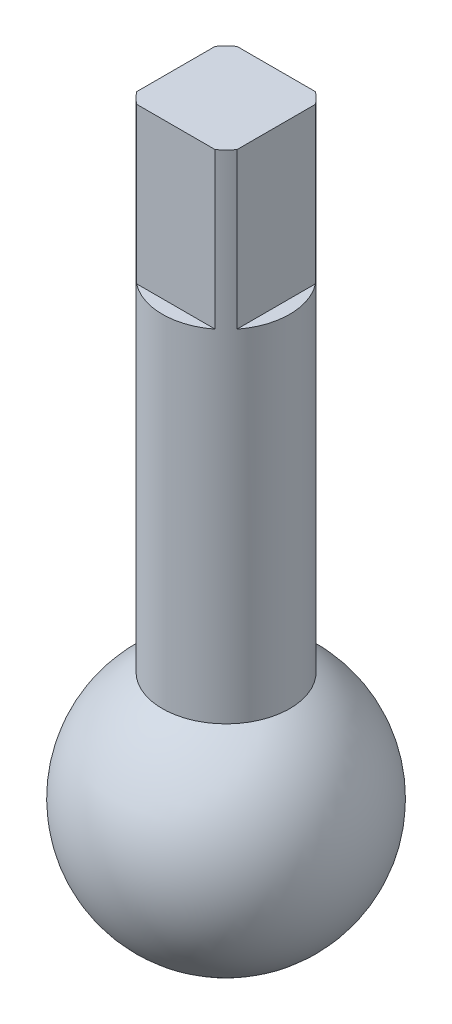
from build123d import *

# Parameters (mm, degrees)
STEM_SHAFT_SKETCH_25_4_R     = 12.7
STEM_SHAFT_25_4_DEPTH        = 90.3
DRIVE_START                  = -31
DRIVE_SQUARE_FLATS_CUT_DEPTH = 31
STEM_START                   = 31
STEM_BOSS_SKETCH_R           = 12.7
STEM_BOSS_31MM_DEPTH         = 31


with BuildPart() as part:
    # Stem Shaft Sketch _25.4 → Stem Shaft _25.4 (new body)
    with BuildSketch(Plane(origin=(0, 0, 0), x_dir=(1, 0, 0), z_dir=(0, 1, 0))):
        with Locations(Location((0, 0, 0), (0, 0, 270))):
            Circle(STEM_SHAFT_SKETCH_25_4_R)
    extrude(amount=STEM_SHAFT_25_4_DEPTH)

    # Drive Square Flats Sketch → Drive Square Flats Cut (cut)
    with BuildSketch(Plane(origin=(0, 90.3, 0), x_dir=(1, 0, 0), z_dir=(0, 1, 0)).offset(DRIVE_START)):
        with BuildLine():
            ThreePointArc((-7.82879301, -10), (0, -12.7), (7.82879301, -10))
            Line((7.82879301, -10), (-7.82879301, -10))
        make_face()
        with BuildLine():
            Line((-10, -7.82879301), (-10, 7.82879301))
            ThreePointArc((-10, 7.82879301), (-12.7, 0), (-10, -7.82879301))
        make_face()
        with BuildLine():
            Line((-7.82879301, 10), (7.82879301, 10))
            ThreePointArc((7.82879301, 10), (0, 12.7), (-7.82879301, 10))
        make_face()
        with BuildLine():
            Line((10, 7.82879301), (10, 0))
            Line((10, 0), (10, -7.82879301))
            ThreePointArc((10, -7.82879301), (12.006040147, -4.140652123), (12.7, 0))
            ThreePointArc((12.7, 0), (12.006040147, 4.140652123), (10, 7.82879301))
        make_face()
    extrude(amount=DRIVE_SQUARE_FLATS_CUT_DEPTH, mode=Mode.SUBTRACT)

    # Stem Boss Sketch → Stem Boss 31mm (add)
    with BuildSketch(Plane.XZ.offset(STEM_START)):
        with Locations(Location((0, 0, 0), (0, 0, 270))):
            Circle(STEM_BOSS_SKETCH_R)
    extrude(amount=-STEM_BOSS_31MM_DEPTH)


with BuildPart() as body_2:
    # Ball Profile Sketch → Valve Ball (revolve)
    with BuildSketch(Plane.XY):
        with BuildLine():
            Line((-25.3, -30.67), (25.3, -30.67))
            ThreePointArc((25.3, -30.67), (0, -55.97), (-25.3, -30.67))
        make_face()
    revolve(axis=Axis((-25.3, -30.67, 0), (1, 0, 0)))

    # Combine1: union part
    add(part.part)


solid = body_2.part
